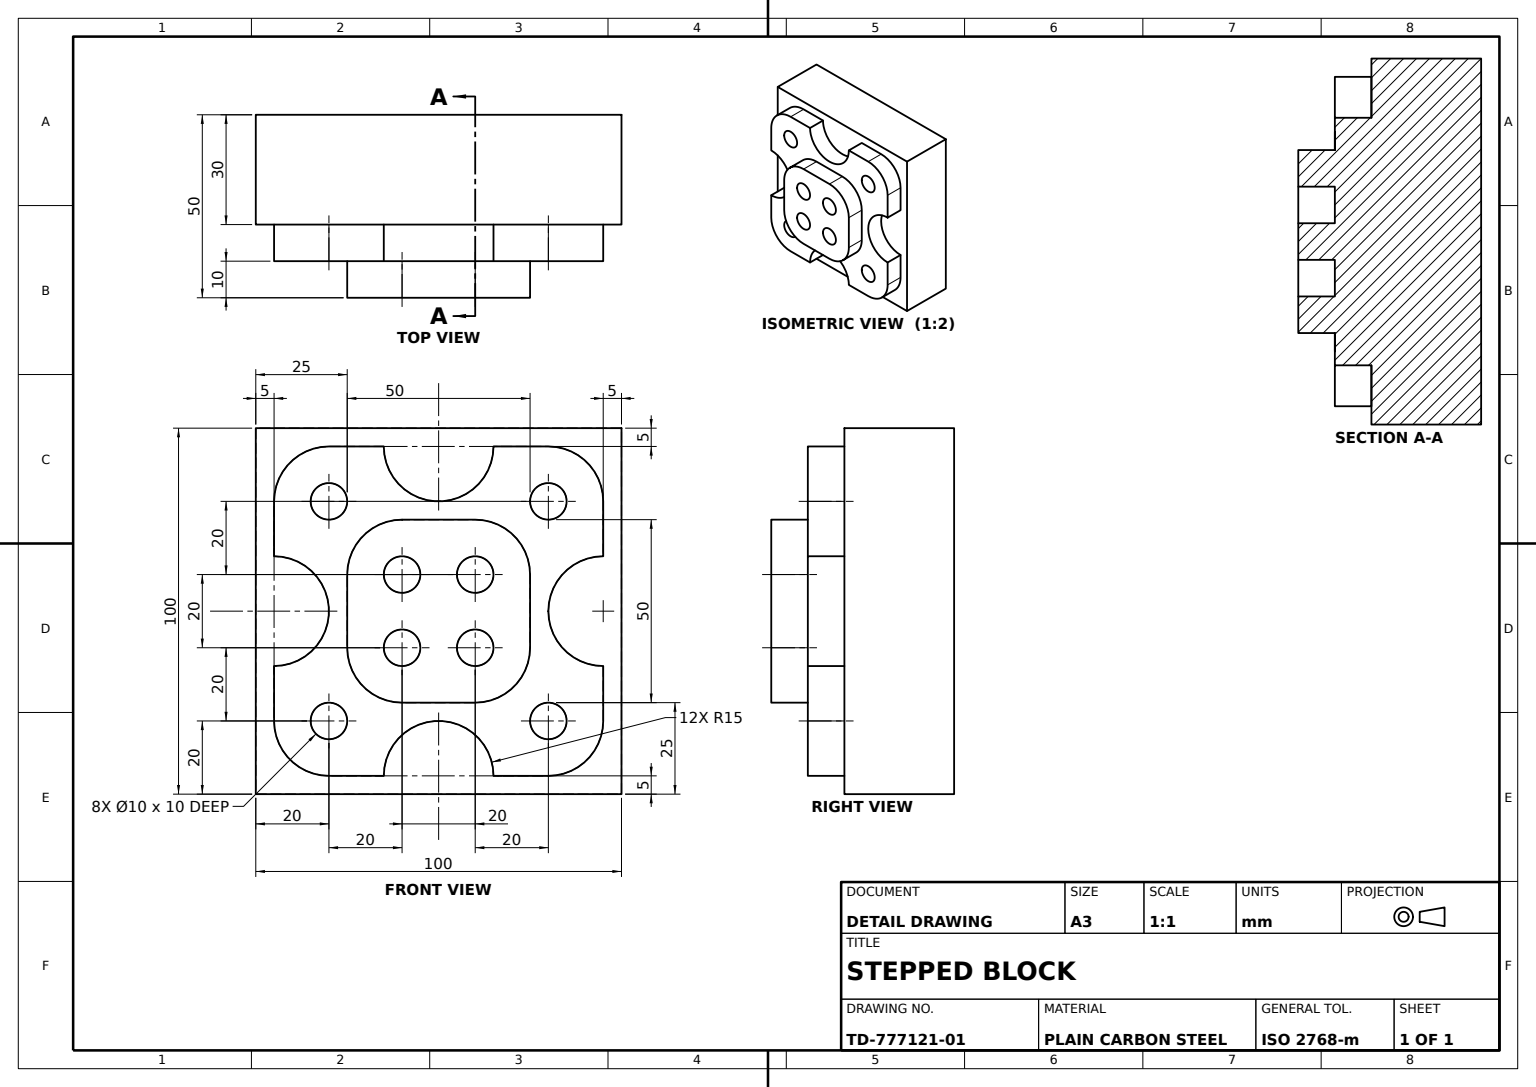
from build123d import *

# Parameters (mm, degrees)
BASE_BLOCK_SKETCH_W         = 100
BASE_BLOCK_SKETCH_H         = 100
BASE_BLOCK_100X100X30_DEPTH = 30
FLANGE_PLATE_DEPTH          = 10
CENTRE_BOSS_DEPTH           = 10
BOSS_HOLES_SKETCH_R         = 5
BOSS_HOLES_4X_10_DEPTH      = 10
FLANGE_HOLES_SKETCH_R       = 5
FLANGE_HOLES_4X_10_DEPTH    = 10


with BuildPart() as part:
    # Base Block Sketch → Base Block 100x100x30 (new body)
    with BuildSketch(Plane.XY):
        with Locations((50, -50)):
            Rectangle(BASE_BLOCK_SKETCH_W, BASE_BLOCK_SKETCH_H)
    extrude(amount=BASE_BLOCK_100X100X30_DEPTH)

    # Flange Plate Sketch → Flange Plate (add)
    with BuildSketch(Plane.XY.offset(30)):
        with BuildLine():
            Line((5, -65), (5, -80))
            ThreePointArc((5, -80), (9.393398282, -90.606601718), (20, -95))
            Line((20, -95), (35, -95))
            ThreePointArc((35, -95), (50, -80), (65, -95))
            Line((65, -95), (80, -95))
            ThreePointArc((80, -95), (90.606601718, -90.606601718), (95, -80))
            Line((95, -80), (95, -65))
            ThreePointArc((95, -65), (80, -50), (95, -35))
            Line((95, -35), (95, -20))
            ThreePointArc((95, -20), (90.606601718, -9.393398282), (80, -5))
            Line((80, -5), (65, -5))
            ThreePointArc((65, -5), (50, -20), (35, -5))
            Line((35, -5), (20, -5))
            ThreePointArc((20, -5), (9.393398282, -9.393398282), (5, -20))
            Line((5, -20), (5, -35))
            ThreePointArc((5, -35), (20, -50), (5, -65))
        make_face()
    extrude(amount=FLANGE_PLATE_DEPTH)

    # Centre Boss Sketch → Centre Boss (add)
    with BuildSketch(Plane.XY.offset(40)):
        with BuildLine():
            Line((25, -40), (25, -60))
            ThreePointArc((25, -60), (29.393398282, -70.606601718), (40, -75))
            Line((40, -75), (60, -75))
            ThreePointArc((60, -75), (70.606601718, -70.606601718), (75, -60))
            Line((75, -60), (75, -40))
            ThreePointArc((75, -40), (70.606601718, -29.393398282), (60, -25))
            Line((60, -25), (40, -25))
            ThreePointArc((40, -25), (29.393398282, -29.393398282), (25, -40))
        make_face()
    extrude(amount=CENTRE_BOSS_DEPTH)

    # Boss Holes Sketch → Boss Holes 4xØ10 (cut)
    with BuildSketch(Plane.XY.offset(50)):
        with Locations((40, -40)):
            Circle(BOSS_HOLES_SKETCH_R)
        with Locations((60, -40)):
            Circle(BOSS_HOLES_SKETCH_R)
        with Locations((60, -60)):
            Circle(BOSS_HOLES_SKETCH_R)
        with Locations((40, -60)):
            Circle(BOSS_HOLES_SKETCH_R)
    extrude(amount=-BOSS_HOLES_4X_10_DEPTH, mode=Mode.SUBTRACT)

    # Flange Holes Sketch → Flange Holes 4xØ10 (cut)
    with BuildSketch(Plane.XY.offset(40)):
        with Locations((20, -20)):
            Circle(FLANGE_HOLES_SKETCH_R)
        with Locations((80, -20)):
            Circle(FLANGE_HOLES_SKETCH_R)
        with Locations((80, -80)):
            Circle(FLANGE_HOLES_SKETCH_R)
        with Locations((20, -80)):
            Circle(FLANGE_HOLES_SKETCH_R)
    extrude(amount=-FLANGE_HOLES_4X_10_DEPTH, mode=Mode.SUBTRACT)


solid = part.part
